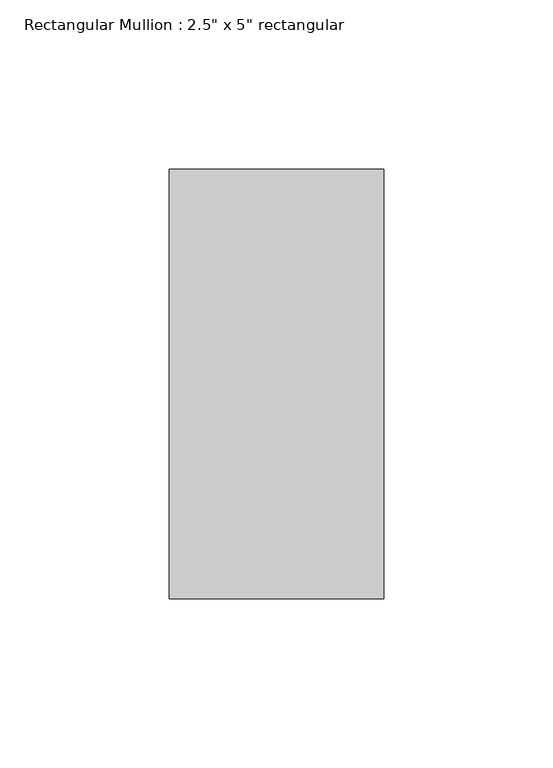
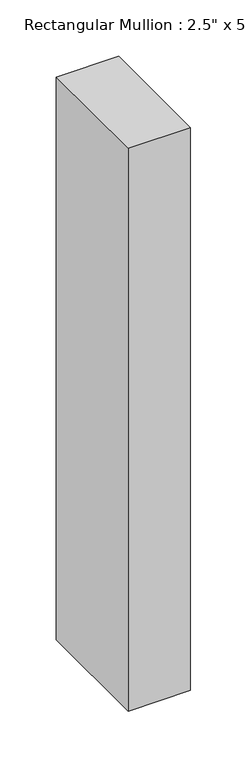
"""IFC4 building model written with IfcOpenShell, lengths in millimetres: member geometry."""

from ifc_helpers import new_model, si_unit, frame, origin, place, context, project, spatial, polyline, outline, extrude, source, transform, mapped, element, save


def member_13f6f031(model_context):
    return source(origin(), model_context, "Body", "SweptSolid", [
        extrude(outline(polyline([(0.0, 63.5), (0.0, -63.5), (-63.5, -63.5), (-63.5, 63.5), (0.0, 63.5)])), frame((0.0, 0.0, -608.6004972), z_axis=(0.0, 0.0, 1.0), x_axis=(1.0, 0.0, 0.0)), (0.0, 0.0, 1.0), 608.6004972),
    ])


if __name__ == "__main__":
    model = new_model("IFC4")
    model_context = context("Model", 3, world=origin())
    ifc_project = project(units=[si_unit("LENGTHUNIT", "METRE", prefix="MILLI")], contexts=[model_context])
    site = spatial("IfcSite", under=ifc_project)
    building = spatial("IfcBuilding", under=site)
    placement = place(None, origin())
    member_shape = member_13f6f031(model_context)
    element("IfcMember", 1, ObjectType="Rectangular Mullion : 2.5\" x 5\" rectangular", at=placement, inside=building, context=model_context, shape_type="MappedRepresentation", body=[
        mapped(member_shape, transform((0.0, 0.0, 0.0), x_axis=(1.0, 0.0, 0.0), y_axis=(0.0, 1.0, 0.0), z_axis=(0.0, 0.0, 1.0))),
    ])
    save(model, "model.ifc")

# Revit data of these elements
# Type "Rectangular Mullion : 2.5\" x 5\" rectangular"
#   built-in parameter 1007304 = 0.416667 (stored number, unit not read)
#   built-in parameter 1007301 = 0.104167 (stored number, unit not read)
#   built-in parameter 1007300 = 0.104167 (stored number, unit not read)
# Element 1 (IfcMember, "Rectangular Mullion : 2.5\" x 5\" rectangular")
#   Materials on its faces: "Aluminum"
# Materials
#   "Aluminum": class "Metal", colour RGB 247 247 247, transparency 0, Description = "Aluminum 6061", Cost = 0
